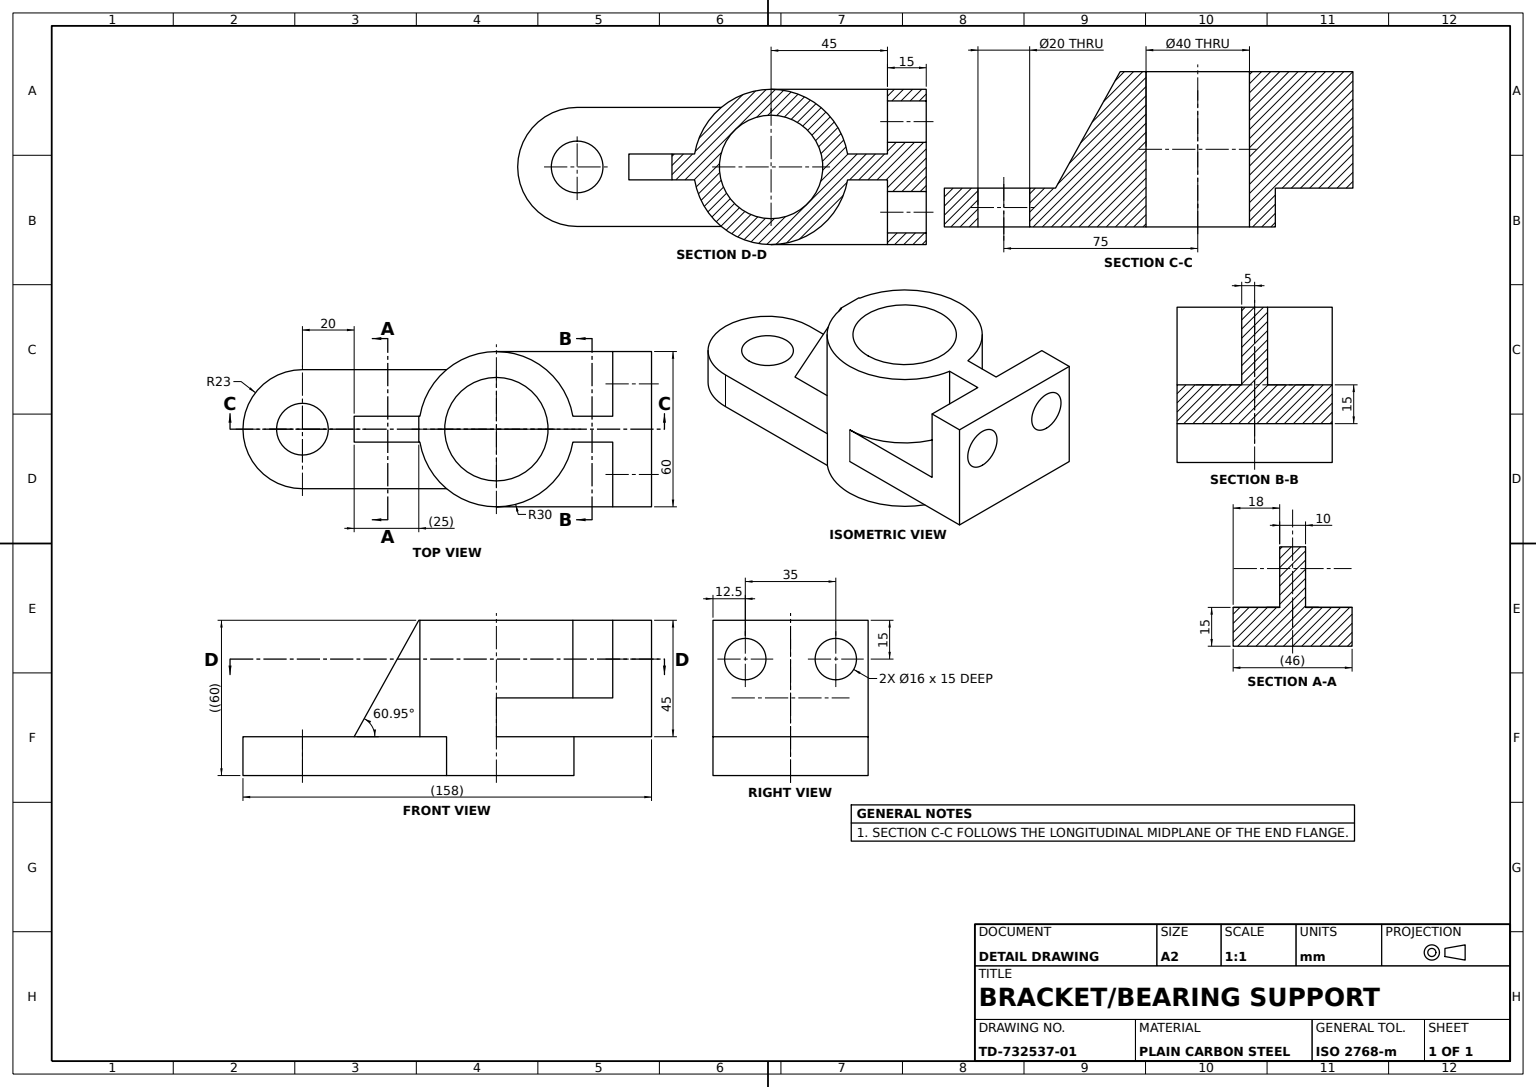
from build123d import *
from build123d.topology import SkipClean

# Parameters (mm, degrees)
BRACKET_BODY_DEPTH      = 30
BRACKET_BODY_SKETCH_W   = 75
BRACKET_BODY_SKETCH_H   = 15
BRACKET_BODY_2_DEPTH    = 30
COLUMN_BORE_SKETCH_R    = 20
COLUMN_BORE_40_DEPTH    = 60
COLUMN_BOSS_SKETCH_R    = 30
COLUMN_BOSS_SKETCH_R_2  = 20
COLUMN_BOSS_60_DEPTH    = 60
BASE_COLLAR_SKETCH_R    = 23
BASE_COLLAR_46_DEPTH    = 15
BODY_TRIM_CUT_SKETCH_R  = 10
BODY_TRIM_CUT_DEPTH     = 112.933015683
SIDE_BLOCK_CUT_SKETCH_R = 8
SIDE_BLOCK_CUT_DEPTH    = 158.952524513
PAD_BOSS_18MM_DEPTH     = 18
SUPPORT_RIB_DEPTH       = 5


with BuildPart() as part:
    # Bracket Body Sketch → Bracket Body (new, symmetric)
    with BuildSketch(Plane.XY):
        Polygon((-60, 15), (-60, 60), (-45, 60), (-45, 30), (0, 30), (0, 15), align=None)
    extrude(amount=BRACKET_BODY_DEPTH, both=True)


with BuildPart() as body_2:
    # Bracket Body Sketch → Bracket Body 2 (new, symmetric)
    with BuildSketch(Plane.XY):
        with Locations((37.5, 7.5)):
            Rectangle(BRACKET_BODY_SKETCH_W, BRACKET_BODY_SKETCH_H)
    extrude(amount=BRACKET_BODY_2_DEPTH, both=True)


with BuildPart() as column_bore_40_tool:
    # Column Bore Sketch → Column Bore Ø40 (new body)
    with BuildSketch(Plane(origin=(0, 0, 0), x_dir=(1, 0, 0), z_dir=(0, 1, 0))):
        Circle(COLUMN_BORE_SKETCH_R)
    extrude(amount=COLUMN_BORE_40_DEPTH)


with BuildPart() as part_1:
    add(part.part)

    # Column Bore Ø40: cut by column_bore_40_tool
    add(column_bore_40_tool.part, mode=Mode.SUBTRACT)



with BuildPart() as body_2_1:
    add(body_2.part)

    # Column Bore Ø40: cut by column_bore_40_tool
    add(column_bore_40_tool.part, mode=Mode.SUBTRACT)


with BuildPart() as part_2:
    add(part_1.part)

    add(body_2_1.part)  # Column Boss Ø60 merges body 2
    # Column Boss Sketch → Column Boss Ø60 (add)
    with BuildSketch(Plane(origin=(0, 0, 0), x_dir=(1, 0, 0), z_dir=(0, 1, 0))):
        with Locations(Location((0, 0, 0), (0, 0, 270))):
            Circle(COLUMN_BOSS_SKETCH_R)
        with Locations(Location((0, 0, 0), (0, 0, 270))):
            Circle(COLUMN_BOSS_SKETCH_R_2, mode=Mode.SUBTRACT)
    extrude(amount=COLUMN_BOSS_60_DEPTH)

    # Base Collar Sketch → Base Collar Ø46 (add)
    with BuildSketch(Plane(origin=(0, 0, 0), x_dir=(1, 0, 0), z_dir=(0, 1, 0))):
        with Locations((75, 0)):
            Circle(BASE_COLLAR_SKETCH_R)
    extrude(amount=BASE_COLLAR_46_DEPTH)

    # Body Trim Cut Sketch → Body Trim Cut (cut, through all)
    with SkipClean():  # the faces are left unmerged after this step: merging them gives an invalid solid
        with BuildSketch(Plane(origin=(0, 15, 0), x_dir=(1, 0, 0), z_dir=(0, 1, 0))):
            with Locations(Location((75, 0, 0), (0, 0, 270))):
                Circle(BODY_TRIM_CUT_SKETCH_R)
            with BuildLine():
                Line((75, 23), (19.261360284, 23))
                ThreePointArc((19.261360284, 23), (10.246950766, 28.19574436), (0, 30))
                Line((0, 30), (75, 30))
                Line((75, 30), (75, 23))
            make_face()
            with BuildLine():
                Line((75, -23), (75, -30))
                Line((75, -30), (0, -30))
                ThreePointArc((0, -30), (10.246950766, -28.19574436), (19.261360284, -23))
                Line((19.261360284, -23), (75, -23))
            make_face()
        extrude(amount=-BODY_TRIM_CUT_DEPTH, mode=Mode.SUBTRACT)

    # Side Block Cut Sketch → Side Block Cut (cut, through all)
    with SkipClean():  # the faces are left unmerged after this step: merging them gives an invalid solid
        with BuildSketch(Plane(origin=(-45, 0, 0), x_dir=(0, 0, -1), z_dir=(1, 0, 0))):
            with Locations(Location((-17.5, 45, 0), (0, 0, 90))):
                Circle(SIDE_BLOCK_CUT_SKETCH_R)
            with Locations(Location((17.5, 45, 0), (0, 0, 270))):
                Circle(SIDE_BLOCK_CUT_SKETCH_R)
        extrude(amount=-SIDE_BLOCK_CUT_DEPTH, mode=Mode.SUBTRACT)

    # Pad Boss Sketch → Pad Boss 18mm (add)
    with SkipClean():  # the faces are left unmerged after this step: merging them gives an invalid solid
        with BuildSketch(Plane(origin=(-45, 0, 0), x_dir=(0, 0, -1), z_dir=(1, 0, 0))):
            Polygon((0, 60), (5, 60), (5, 30), (-5, 30), (-5, 60), align=None)
        extrude(amount=PAD_BOSS_18MM_DEPTH)

    # Support Rib Sketch → Support Rib (add, symmetric)
    with BuildSketch(Plane.XY):
        Polygon((30, 15), (55, 15), (30, 60), (20, 60), (20, 15), align=None)
    extrude(amount=SUPPORT_RIB_DEPTH, both=True)


solid = part_2.part
